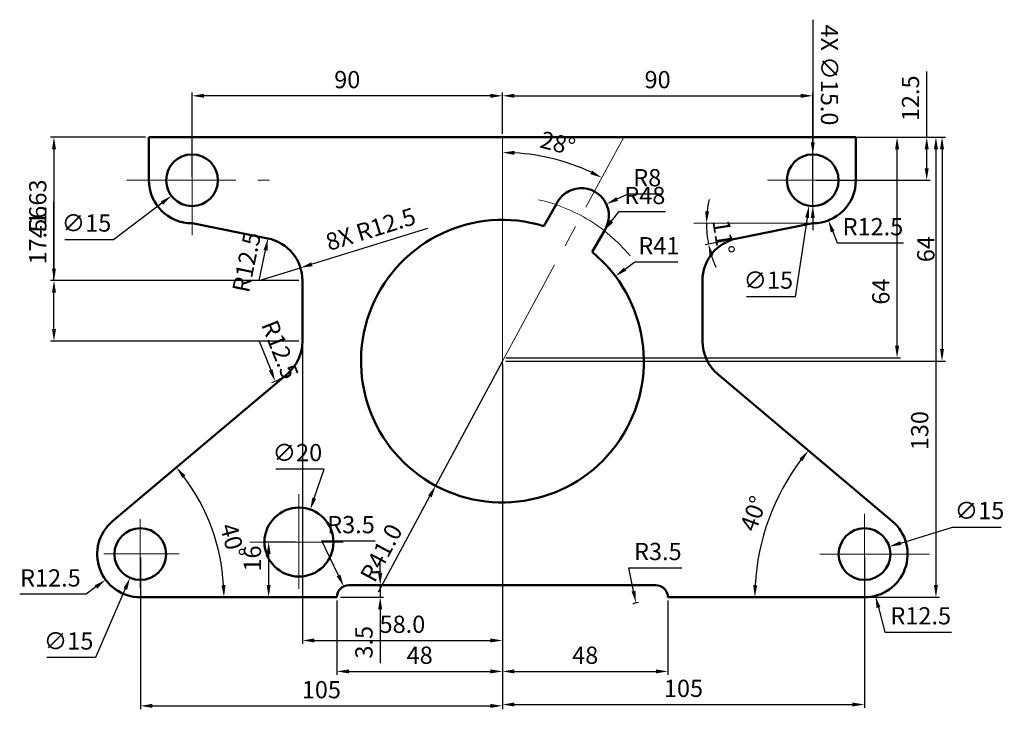
# Model space of a CAD drawing. Units: millimetres. Extents: x 3173 to 3458, y 769 to 969.
import ezdxf

# ---------------------------------------------------------------- set-up
doc = ezdxf.new("R2010")
doc.units = ezdxf.units.MM
doc.linetypes.add('CENTER', pattern=[50.8, 31.75, -6.35, 6.35, -6.35])
for name, color, linetype, lineweight in [('M-CNTR', 7, 'CENTER', 18), ('M-CONS', 8, 'Continuous', 13), ('M-DIMS', 3, 'Continuous', 25), ('M-OUTL', 7, 'Continuous', 50)]:
    doc.layers.add(name, color=color, linetype=linetype, lineweight=lineweight)
doc.styles.get("Standard").update_dxf_attribs({"font": 'arial.ttf'})
doc.dimstyles.new('AM_ISO$0', dxfattribs={"dimtxt": 5, "dimasz": 3.5, "dimexe": 1, "dimexo": 1, "dimgap": 1.5, "dimtad": 1, "dimdsep": 46, "dimtxsty": 'Standard', "dimcen": 0, "dimclrd": 256, "dimclre": 256, "dimclrt": 2, "dimadec": 0, "dimazin": 2, "dimtp": 0.1, "dimtm": 0.1, "dimtfac": 0.71, "dimtmove": 0, "dimatfit": 3, "dimfxl": 1, "dimlwd": -1, "dimlwe": -1, "dimarcsym": 1})
doc.dimstyles.new('AM_ISO$2', dxfattribs={"dimtxt": 5, "dimasz": 3.5, "dimexe": 1, "dimexo": 1, "dimgap": 1.5, "dimtad": 1, "dimdsep": 46, "dimtxsty": 'Standard', "dimcen": 0, "dimclrd": 256, "dimclre": 256, "dimclrt": 2, "dimadec": 0, "dimazin": 2, "dimtp": 0.1, "dimtm": 0.1, "dimtfac": 0.71, "dimtmove": 0, "dimatfit": 3, "dimfxl": 1, "dimlwd": -1, "dimlwe": -1, "dimarcsym": 1})
doc.dimstyles.new('AM_ISO$3', dxfattribs={"dimtxt": 5, "dimasz": 3.5, "dimexe": 1, "dimexo": 1, "dimgap": 1.5, "dimtad": 1, "dimtoh": 1, "dimdsep": 46, "dimtxsty": 'Standard', "dimcen": 0, "dimclrd": 256, "dimclre": 256, "dimclrt": 2, "dimadec": 0, "dimazin": 2, "dimtp": 0.1, "dimtm": 0.1, "dimtfac": 0.71, "dimtofl": 0, "dimtmove": 0, "dimatfit": 0, "dimfxl": 1, "dimlwd": -1, "dimlwe": -1, "dimarcsym": 1})
doc.dimstyles.new('AM_ISO$4', dxfattribs={"dimtxt": 5, "dimasz": 3.5, "dimexe": 1, "dimexo": 1, "dimgap": 1.5, "dimtad": 1, "dimtoh": 1, "dimdsep": 46, "dimtxsty": 'Standard', "dimcen": 0, "dimclrd": 256, "dimclre": 256, "dimclrt": 2, "dimadec": 0, "dimazin": 2, "dimtp": 0.1, "dimtm": 0.1, "dimtfac": 0.71, "dimtofl": 0, "dimtmove": 0, "dimatfit": 0, "dimfxl": 1, "dimlwd": -1, "dimlwe": -1, "dimarcsym": 1})

# ---------------------------------------------------------------- blocks, each defined once
blk = doc.blocks.new('*D3')
at = {"layer": 'Defpoints', "color": 0, "transparency": 16777216}
for p in [(3375.11, 866.04), (3392.94, 831.01), (3425.73, 823.34), (3360.67, 801.29), (3417.67, 801.29)]:
    blk.add_point(p, dxfattribs=at)
at = {"layer": 'M-DIMS', "color": 0, "linetype": 'ByBlock', "transparency": 16777216}
blk.add_arc((3451.87, 801.29), 66, 142.8895, 176.9613, dxfattribs=at)
at = {"layer": 'M-DIMS', "color": 0, "transparency": 16777216}
for points in [[(3398.78, 841.48), (3399.69, 840.75), (3401.42, 843.85)], [(3386.55, 804.77), (3385.38, 804.8), (3385.87, 801.29)]]:
    blk.add_solid(points, dxfattribs=at)
at = {"layer": 'M-DIMS', "color": 0, "transparency": 16777216, "insert": (3386.07, 825.34), "char_height": 5, "attachment_point": 5, "rotation": 69.9254}
blk.add_mtext('40°', dxfattribs=at)
blk = doc.blocks.new('*D4')
at = {"layer": 'Defpoints', "color": 0, "transparency": 16777216}
for p in [(3250.23, 866.04), (3225.65, 827.61), (3199.61, 823.34), (3207.67, 801.29), (3264.67, 801.29)]:
    blk.add_point(p, dxfattribs=at)
at = {"layer": 'M-DIMS', "color": 0, "linetype": 'ByBlock', "transparency": 16777216}
blk.add_arc((3173.46, 801.29), 58.45, 3.4314, 36.7177, dxfattribs=at)
at = {"layer": 'M-DIMS', "color": 0, "transparency": 16777216}
for points in [[(3219.86, 835.87), (3220.77, 836.6), (3218.14, 838.98)], [(3232.39, 804.81), (3231.22, 804.77), (3231.91, 801.29)]]:
    blk.add_solid(points, dxfattribs=at)
at = {"layer": 'M-DIMS', "color": 0, "transparency": 16777216, "insert": (3233.83, 817.5), "char_height": 5, "attachment_point": 5, "rotation": 285.0268}
blk.add_mtext('40°', dxfattribs=at)
blk = doc.blocks.new('*D5')
at = {"layer": 'Defpoints', "color": 0, "transparency": 16777216}
for p in [(3368.19, 909.79), (3402.67, 909.79), (3402.67, 909.79), (3371.9, 907.77), (3380.72, 905.42)]:
    blk.add_point(p, dxfattribs=at)
at = {"layer": 'M-DIMS', "color": 0, "linetype": 'ByBlock', "transparency": 16777216}
blk.add_line((3379.74, 905.22), (3371.44, 903.57), dxfattribs=at)
for start, end in [(166.9868, 173.4934), (180, 191.2657), (197.7723, 204.2789)]:
    blk.add_arc((3402.67, 909.79), 30.84, start, end, dxfattribs=at)
at = {"layer": 'M-DIMS', "color": 0, "transparency": 16777216}
for points in [[(3372.61, 913.25), (3371.45, 913.32), (3371.83, 909.79)], [(3372.74, 900.23), (3373.87, 900.52), (3372.42, 903.77)]]:
    blk.add_solid(points, dxfattribs=at)
at = {"layer": 'M-DIMS', "color": 0, "transparency": 16777216, "insert": (3376.16, 905.64), "char_height": 5, "attachment_point": 5, "rotation": 278.895}
blk.add_mtext('11°', dxfattribs=at)
blk = doc.blocks.new('*D6')
at = {"layer": 'Defpoints', "color": 0, "transparency": 16777216}
for p in [(3244.68, 905.41), (3242.17, 893.16)]:
    blk.add_point(p, dxfattribs=at)
at = {"layer": 'M-DIMS', "color": 0, "linetype": 'ByBlock', "transparency": 16777216}
blk.add_line((3242.17, 893.16), (3243.97, 901.98), dxfattribs=at)
at = {"layer": 'M-DIMS', "color": 0, "transparency": 16777216}
blk.add_solid([(3243.4, 902.09), (3244.55, 901.86), (3244.68, 905.41)], dxfattribs=at)
at = {"layer": 'M-DIMS', "color": 0, "transparency": 16777216, "insert": (3239.1, 898.38), "char_height": 5, "attachment_point": 5, "rotation": 78.4102}
blk.add_mtext('R12.5', dxfattribs=at)
blk = doc.blocks.new('*D7')
at = {"layer": 'Defpoints', "color": 0, "transparency": 16777216}
for p in [(3242.17, 875.6), (3246.75, 863.97)]:
    blk.add_point(p, dxfattribs=at)
at = {"layer": 'M-DIMS', "color": 0, "linetype": 'ByBlock', "transparency": 16777216}
blk.add_line((3242.17, 875.6), (3245.47, 867.23), dxfattribs=at)
blk.add_arc((3242.17, 875.6), 12.5, 286.9476, 305.5655, dxfattribs=at)
at = {"layer": 'M-DIMS', "color": 0, "transparency": 16777216}
blk.add_solid([(3246.01, 867.44), (3244.93, 867.01), (3246.75, 863.97)], dxfattribs=at)
at = {"layer": 'M-DIMS', "color": 0, "transparency": 16777216, "insert": (3247.59, 872.9), "char_height": 5, "attachment_point": 5, "rotation": 291.5312}
blk.add_mtext('R12.5', dxfattribs=at)
blk = doc.blocks.new('*D8')
at = {"layer": 'Defpoints', "color": 0, "transparency": 16777216}
for p in [(3351.39, 799.65), (3352.09, 796.22)]:
    blk.add_point(p, dxfattribs=at)
at = {"layer": 'M-DIMS', "color": 0, "linetype": 'ByBlock', "transparency": 16777216}
for p, q in [((3350.68, 803.07), (3349.28, 809.86)), ((3349.28, 809.86), (3364.7, 809.86))]:
    blk.add_line(p, q, dxfattribs=at)
blk.add_arc((3352.09, 796.22), 3.5, 90, 118.0492, dxfattribs=at)
at = {"layer": 'M-DIMS', "color": 0, "transparency": 16777216}
blk.add_solid([(3351.25, 803.19), (3350.11, 802.96), (3351.39, 799.65)], dxfattribs=at)
at = {"layer": 'M-DIMS', "color": 0, "transparency": 16777216, "insert": (3357.74, 813.91), "char_height": 5, "attachment_point": 5}
blk.add_mtext('R3.5', dxfattribs=at)
blk = doc.blocks.new('*D9')
at = {"layer": 'Defpoints', "color": 0, "transparency": 16777216}
for p in [(3266.65, 804.44), (3268.17, 801.29)]:
    blk.add_point(p, dxfattribs=at)
at = {"layer": 'M-DIMS', "color": 0, "linetype": 'ByBlock', "transparency": 16777216}
for p, q in [((3265.13, 807.6), (3260.3, 817.65)), ((3260.3, 817.65), (3275.73, 817.65))]:
    blk.add_line(p, q, dxfattribs=at)
at = {"layer": 'M-DIMS', "color": 0, "transparency": 16777216}
blk.add_solid([(3265.66, 807.85), (3264.61, 807.35), (3266.65, 804.44)], dxfattribs=at)
at = {"layer": 'M-DIMS', "color": 0, "transparency": 16777216, "insert": (3268.76, 821.7), "char_height": 5, "attachment_point": 5}
blk.add_mtext('R3.5', dxfattribs=at)
blk = doc.blocks.new('*D10')
at = {"layer": 'Defpoints', "color": 0, "transparency": 16777216}
for p in [(3342.79, 915.37), (3335.54, 911.99)]:
    blk.add_point(p, dxfattribs=at)
at = {"layer": 'M-DIMS', "color": 0, "linetype": 'ByBlock', "transparency": 16777216}
for p, q in [((3345.96, 916.85), (3349.14, 918.32)), ((3349.14, 918.32), (3358.71, 918.32))]:
    blk.add_line(p, q, dxfattribs=at)
at = {"layer": 'M-DIMS', "color": 0, "transparency": 16777216}
blk.add_solid([(3345.72, 917.37), (3346.21, 916.32), (3342.79, 915.37)], dxfattribs=at)
at = {"layer": 'M-DIMS', "color": 0, "transparency": 16777216, "insert": (3354.67, 922.38), "char_height": 5, "attachment_point": 5}
blk.add_mtext('R8', dxfattribs=at)
blk = doc.blocks.new('*D11')
at = {"layer": 'Defpoints', "color": 0, "transparency": 16777216}
for p in [(3345.45, 894.41), (3312.67, 869.79)]:
    blk.add_point(p, dxfattribs=at)
at = {"layer": 'M-DIMS', "color": 0, "linetype": 'ByBlock', "transparency": 16777216}
for p, q in [((3348.25, 896.52), (3351.05, 898.62)), ((3351.05, 898.62), (3363.53, 898.62))]:
    blk.add_line(p, q, dxfattribs=at)
at = {"layer": 'M-DIMS', "color": 0, "transparency": 16777216}
blk.add_solid([(3347.9, 896.98), (3348.6, 896.05), (3345.45, 894.41)], dxfattribs=at)
at = {"layer": 'M-DIMS', "color": 0, "transparency": 16777216, "insert": (3358.04, 902.63), "char_height": 5, "attachment_point": 5}
blk.add_mtext('R41', dxfattribs=at)
blk = doc.blocks.new('*D12')
at = {"layer": 'Defpoints', "color": 0, "transparency": 16777216}
for p in [(3342.18, 907.65), (3312.67, 869.79)]:
    blk.add_point(p, dxfattribs=at)
at = {"layer": 'M-DIMS', "color": 0, "linetype": 'ByBlock', "transparency": 16777216}
for p, q in [((3344.33, 910.41), (3346.48, 913.17)), ((3346.48, 913.17), (3359.94, 913.17))]:
    blk.add_line(p, q, dxfattribs=at)
at = {"layer": 'M-DIMS', "color": 0, "transparency": 16777216}
blk.add_solid([(3343.87, 910.77), (3344.79, 910.05), (3342.18, 907.65)], dxfattribs=at)
at = {"layer": 'M-DIMS', "color": 0, "transparency": 16777216, "insert": (3353.96, 917.22), "char_height": 5, "attachment_point": 5}
blk.add_mtext('R48', dxfattribs=at)
blk = doc.blocks.new('*D13')
at = {"layer": 'Defpoints', "color": 0, "transparency": 16777216}
for p in [(3417.67, 813.79), (3420.82, 801.7)]:
    blk.add_point(p, dxfattribs=at)
at = {"layer": 'M-DIMS', "color": 0, "linetype": 'ByBlock', "transparency": 16777216}
for p, q in [((3421.71, 798.31), (3423.57, 791.19)), ((3423.57, 791.19), (3442.88, 791.19))]:
    blk.add_line(p, q, dxfattribs=at)
at = {"layer": 'M-DIMS', "color": 0, "transparency": 16777216}
blk.add_solid([(3422.27, 798.46), (3421.14, 798.16), (3420.82, 801.7)], dxfattribs=at)
at = {"layer": 'M-DIMS', "color": 0, "transparency": 16777216, "insert": (3433.97, 795.25), "char_height": 5, "attachment_point": 5}
blk.add_mtext('R12.5', dxfattribs=at)
blk = doc.blocks.new('*D14')
at = {"layer": 'Defpoints', "color": 0, "transparency": 16777216}
for p in [(3207.67, 813.79), (3197.62, 806.35)]:
    blk.add_point(p, dxfattribs=at)
at = {"layer": 'M-DIMS', "color": 0, "linetype": 'ByBlock', "transparency": 16777216}
for p, q in [((3194.81, 804.27), (3192, 802.19)), ((3192, 802.19), (3172.69, 802.19))]:
    blk.add_line(p, q, dxfattribs=at)
at = {"layer": 'M-DIMS', "color": 0, "transparency": 16777216}
blk.add_solid([(3194.46, 804.74), (3195.16, 803.8), (3197.62, 806.35)], dxfattribs=at)
at = {"layer": 'M-DIMS', "color": 0, "transparency": 16777216, "insert": (3181.59, 806.24), "char_height": 5, "attachment_point": 5}
blk.add_mtext('R12.5', dxfattribs=at)
blk = doc.blocks.new('*D15')
at = {"layer": 'Defpoints', "color": 0, "transparency": 16777216}
for p in [(3402.67, 922.29), (3407.18, 910.63)]:
    blk.add_point(p, dxfattribs=at)
at = {"layer": 'M-DIMS', "color": 0, "linetype": 'ByBlock', "transparency": 16777216}
for p, q in [((3408.44, 907.37), (3409.71, 904.1)), ((3409.71, 904.1), (3429.02, 904.1))]:
    blk.add_line(p, q, dxfattribs=at)
at = {"layer": 'M-DIMS', "color": 0, "transparency": 16777216}
blk.add_solid([(3408.99, 907.58), (3407.9, 907.16), (3407.18, 910.63)], dxfattribs=at)
at = {"layer": 'M-DIMS', "color": 0, "transparency": 16777216, "insert": (3420.11, 908.16), "char_height": 5, "attachment_point": 5}
blk.add_mtext('R12.5', dxfattribs=at)
blk = doc.blocks.new('*D16')
at = {"layer": 'Defpoints', "color": 0, "transparency": 16777216}
for p in [(3402.67, 946.79), (3312.67, 934.79), (3402.67, 922.29)]:
    blk.add_point(p, dxfattribs=at)
at = {"layer": 'M-DIMS', "color": 0, "linetype": 'ByBlock', "transparency": 16777216}
for p, q in [((3312.67, 935.79), (3312.67, 947.79)), ((3316.17, 946.79), (3399.17, 946.79)), ((3402.67, 923.29), (3402.67, 947.79))]:
    blk.add_line(p, q, dxfattribs=at)
at = {"layer": 'M-DIMS', "color": 0, "transparency": 16777216}
for points in [[(3316.17, 947.37), (3316.17, 946.21), (3312.67, 946.79)], [(3399.17, 947.37), (3399.17, 946.21), (3402.67, 946.79)]]:
    blk.add_solid(points, dxfattribs=at)
at = {"layer": 'M-DIMS', "color": 0, "transparency": 16777216, "insert": (3357.67, 950.84), "char_height": 5, "attachment_point": 5}
blk.add_mtext('90', dxfattribs=at)
blk = doc.blocks.new('*D17')
at = {"layer": 'Defpoints', "color": 0, "transparency": 16777216}
for p in [(3222.67, 946.79), (3312.67, 934.79), (3222.67, 922.29)]:
    blk.add_point(p, dxfattribs=at)
at = {"layer": 'M-DIMS', "color": 0, "linetype": 'ByBlock', "transparency": 16777216}
for p, q in [((3222.67, 923.29), (3222.67, 947.79)), ((3309.17, 946.79), (3226.17, 946.79)), ((3312.67, 935.79), (3312.67, 947.79))]:
    blk.add_line(p, q, dxfattribs=at)
at = {"layer": 'M-DIMS', "color": 0, "transparency": 16777216}
for points in [[(3226.17, 947.37), (3226.17, 946.21), (3222.67, 946.79)], [(3309.17, 947.37), (3309.17, 946.21), (3312.67, 946.79)]]:
    blk.add_solid(points, dxfattribs=at)
at = {"layer": 'M-DIMS', "color": 0, "transparency": 16777216, "insert": (3267.67, 950.84), "char_height": 5, "attachment_point": 5}
blk.add_mtext('90', dxfattribs=at)
blk = doc.blocks.new('*D18')
at = {"layer": 'Defpoints', "color": 0, "transparency": 16777216}
for p in [(3256.95, 826.74), (3250.38, 807.84)]:
    blk.add_point(p, dxfattribs=at)
at = {"layer": 'M-DIMS', "color": 0, "linetype": 'ByBlock', "transparency": 16777216}
for p, q in [((3261, 838.41), (3246.92, 838.41)), ((3258.1, 830.04), (3261, 838.41))]:
    blk.add_line(p, q, dxfattribs=at)
at = {"layer": 'M-DIMS', "color": 0, "transparency": 16777216}
blk.add_solid([(3257.55, 830.23), (3258.65, 829.85), (3256.95, 826.74)], dxfattribs=at)
at = {"layer": 'M-DIMS', "color": 0, "transparency": 16777216, "insert": (3253.21, 842.6), "char_height": 5, "attachment_point": 5}
blk.add_mtext('∅20', dxfattribs=at)
blk = doc.blocks.new('*D19')
at = {"layer": 'Defpoints', "color": 0, "transparency": 16777216}
for p in [(3253.67, 817.29), (3244.88, 801.29), (3253.63, 801.29)]:
    blk.add_point(p, dxfattribs=at)
at = {"layer": 'M-DIMS', "color": 0, "linetype": 'ByBlock', "transparency": 16777216}
for p, q in [((3252.67, 817.29), (3243.88, 817.29)), ((3244.88, 813.79), (3244.88, 804.79)), ((3252.63, 801.29), (3243.88, 801.29))]:
    blk.add_line(p, q, dxfattribs=at)
at = {"layer": 'M-DIMS', "color": 0, "transparency": 16777216}
for points in [[(3244.29, 813.79), (3245.46, 813.79), (3244.88, 817.29)], [(3244.29, 804.79), (3245.46, 804.79), (3244.88, 801.29)]]:
    blk.add_solid(points, dxfattribs=at)
at = {"layer": 'M-DIMS', "color": 0, "transparency": 16777216, "insert": (3240.82, 812.52), "char_height": 5, "attachment_point": 5, "rotation": 90}
blk.add_mtext('16', dxfattribs=at)
blk = doc.blocks.new('*D20')
at = {"layer": 'Defpoints', "color": 0, "transparency": 16777216}
for p in [(3271.93, 804.79), (3277.22, 804.79), (3264.67, 801.29)]:
    blk.add_point(p, dxfattribs=at)
at = {"layer": 'M-DIMS', "color": 0, "linetype": 'ByBlock', "transparency": 16777216}
for p, q in [((3277.22, 808.29), (3277.22, 811.79)), ((3272.93, 804.79), (3278.22, 804.79)), ((3277.22, 804.79), (3277.22, 801.29)), ((3265.67, 801.29), (3278.22, 801.29)), ((3277.22, 797.79), (3277.22, 782.15))]:
    blk.add_line(p, q, dxfattribs=at)
at = {"layer": 'M-DIMS', "color": 0, "transparency": 16777216}
for points in [[(3276.63, 808.29), (3277.8, 808.29), (3277.22, 804.79)], [(3276.63, 797.79), (3277.8, 797.79), (3277.22, 801.29)]]:
    blk.add_solid(points, dxfattribs=at)
at = {"layer": 'M-DIMS', "color": 0, "transparency": 16777216, "insert": (3273.16, 788.22), "char_height": 5, "attachment_point": 5, "rotation": 90}
blk.add_mtext('3.5', dxfattribs=at)
blk = doc.blocks.new('*D21')
at = {"layer": 'Defpoints', "color": 0, "transparency": 16777216}
for p in [(3312.67, 804.79), (3360.67, 801.29), (3360.67, 779.76)]:
    blk.add_point(p, dxfattribs=at)
at = {"layer": 'M-DIMS', "color": 0, "linetype": 'ByBlock', "transparency": 16777216}
for p, q in [((3312.67, 803.79), (3312.67, 778.76)), ((3360.67, 800.29), (3360.67, 778.76)), ((3316.17, 779.76), (3357.17, 779.76))]:
    blk.add_line(p, q, dxfattribs=at)
at = {"layer": 'M-DIMS', "color": 0, "transparency": 16777216}
for points in [[(3316.17, 780.34), (3316.17, 779.18), (3312.67, 779.76)], [(3357.17, 780.34), (3357.17, 779.18), (3360.67, 779.76)]]:
    blk.add_solid(points, dxfattribs=at)
at = {"layer": 'M-DIMS', "color": 0, "transparency": 16777216, "insert": (3336.67, 783.81), "char_height": 5, "attachment_point": 5}
blk.add_mtext('48', dxfattribs=at)
blk = doc.blocks.new('*D22')
at = {"layer": 'Defpoints', "color": 0, "transparency": 16777216}
for p in [(3312.67, 804.79), (3264.67, 801.29), (3312.67, 779.76)]:
    blk.add_point(p, dxfattribs=at)
at = {"layer": 'M-DIMS', "color": 0, "linetype": 'ByBlock', "transparency": 16777216}
for p, q in [((3312.67, 803.79), (3312.67, 778.76)), ((3264.67, 800.29), (3264.67, 778.76)), ((3268.17, 779.76), (3309.17, 779.76))]:
    blk.add_line(p, q, dxfattribs=at)
at = {"layer": 'M-DIMS', "color": 0, "transparency": 16777216}
for points in [[(3268.17, 780.34), (3268.17, 779.18), (3264.67, 779.76)], [(3309.17, 780.34), (3309.17, 779.18), (3312.67, 779.76)]]:
    blk.add_solid(points, dxfattribs=at)
at = {"layer": 'M-DIMS', "color": 0, "transparency": 16777216, "insert": (3288.67, 783.81), "char_height": 5, "attachment_point": 5}
blk.add_mtext('48', dxfattribs=at)
blk = doc.blocks.new('*D23')
at = {"layer": 'Defpoints', "color": 0, "transparency": 16777216}
for p in [(3207.67, 813.79), (3312.67, 804.79), (3312.67, 769.76)]:
    blk.add_point(p, dxfattribs=at)
at = {"layer": 'M-DIMS', "color": 0, "linetype": 'ByBlock', "transparency": 16777216}
for p, q in [((3207.67, 812.79), (3207.67, 768.76)), ((3312.67, 803.79), (3312.67, 768.76)), ((3211.17, 769.76), (3309.17, 769.76))]:
    blk.add_line(p, q, dxfattribs=at)
at = {"layer": 'M-DIMS', "color": 0, "transparency": 16777216}
for points in [[(3211.17, 770.34), (3211.17, 769.18), (3207.67, 769.76)], [(3309.17, 770.34), (3309.17, 769.18), (3312.67, 769.76)]]:
    blk.add_solid(points, dxfattribs=at)
at = {"layer": 'M-DIMS', "color": 0, "transparency": 16777216, "insert": (3260.17, 773.81), "char_height": 5, "attachment_point": 5}
blk.add_mtext('105', dxfattribs=at)
blk = doc.blocks.new('*D24')
at = {"layer": 'Defpoints', "color": 0, "transparency": 16777216}
for p in [(3417.67, 813.79), (3312.67, 804.79), (3417.67, 770.15)]:
    blk.add_point(p, dxfattribs=at)
at = {"layer": 'M-DIMS', "color": 0, "linetype": 'ByBlock', "transparency": 16777216}
for p, q in [((3417.67, 812.79), (3417.67, 769.15)), ((3312.67, 803.79), (3312.67, 769.15)), ((3316.17, 770.15), (3414.17, 770.15))]:
    blk.add_line(p, q, dxfattribs=at)
at = {"layer": 'M-DIMS', "color": 0, "transparency": 16777216}
for points in [[(3316.17, 770.73), (3316.17, 769.57), (3312.67, 770.15)], [(3414.17, 770.73), (3414.17, 769.57), (3417.67, 770.15)]]:
    blk.add_solid(points, dxfattribs=at)
at = {"layer": 'M-DIMS', "color": 0, "transparency": 16777216, "insert": (3365.17, 774.2), "char_height": 5, "attachment_point": 5}
blk.add_mtext('105', dxfattribs=at)
blk = doc.blocks.new('*D25')
at = {"layer": 'Defpoints', "color": 0, "transparency": 16777216}
for p in [(3415.17, 934.79), (3312.67, 869.79), (3440.14, 869.79)]:
    blk.add_point(p, dxfattribs=at)
at = {"layer": 'M-DIMS', "color": 0, "linetype": 'ByBlock', "transparency": 16777216}
for p, q in [((3416.17, 934.79), (3441.14, 934.79)), ((3440.14, 931.29), (3440.14, 873.29)), ((3313.67, 869.79), (3441.14, 869.79))]:
    blk.add_line(p, q, dxfattribs=at)
at = {"layer": 'M-DIMS', "color": 0, "transparency": 16777216}
for points in [[(3439.56, 931.29), (3440.72, 931.29), (3440.14, 934.79)], [(3439.56, 873.29), (3440.72, 873.29), (3440.14, 869.79)]]:
    blk.add_solid(points, dxfattribs=at)
at = {"layer": 'M-DIMS', "color": 0, "transparency": 16777216, "insert": (3436.09, 902.29), "char_height": 5, "attachment_point": 5, "rotation": 90}
blk.add_mtext('64', dxfattribs=at)
blk = doc.blocks.new('*D26')
at = {"layer": 'Defpoints', "color": 0, "transparency": 16777216}
for p in [(3415.17, 934.79), (3427.11, 934.79), (3312.67, 870.79)]:
    blk.add_point(p, dxfattribs=at)
at = {"layer": 'M-DIMS', "color": 0, "linetype": 'ByBlock', "transparency": 16777216}
for p, q in [((3416.17, 934.79), (3428.11, 934.79)), ((3427.11, 874.29), (3427.11, 931.29)), ((3313.67, 870.79), (3428.11, 870.79))]:
    blk.add_line(p, q, dxfattribs=at)
at = {"layer": 'M-DIMS', "color": 0, "transparency": 16777216}
for points in [[(3426.53, 931.29), (3427.7, 931.29), (3427.11, 934.79)], [(3426.53, 874.29), (3427.7, 874.29), (3427.11, 870.79)]]:
    blk.add_solid(points, dxfattribs=at)
at = {"layer": 'M-DIMS', "color": 0, "transparency": 16777216, "insert": (3423.06, 889.97), "char_height": 5, "attachment_point": 5, "rotation": 90}
blk.add_mtext('64', dxfattribs=at)
blk = doc.blocks.new('*D27')
at = {"layer": 'Defpoints', "color": 0, "transparency": 16777216}
for p in [(3415.17, 934.79), (3407.81, 801.29), (3438.38, 801.29)]:
    blk.add_point(p, dxfattribs=at)
at = {"layer": 'M-DIMS', "color": 0, "linetype": 'ByBlock', "transparency": 16777216}
for p, q in [((3416.17, 934.79), (3439.38, 934.79)), ((3438.38, 931.29), (3438.38, 804.79)), ((3408.81, 801.29), (3439.38, 801.29))]:
    blk.add_line(p, q, dxfattribs=at)
at = {"layer": 'M-DIMS', "color": 0, "transparency": 16777216}
for points in [[(3437.79, 931.29), (3438.96, 931.29), (3438.38, 934.79)], [(3437.79, 804.79), (3438.96, 804.79), (3438.38, 801.29)]]:
    blk.add_solid(points, dxfattribs=at)
at = {"layer": 'M-DIMS', "color": 0, "transparency": 16777216, "insert": (3434.32, 849.62), "char_height": 5, "attachment_point": 5, "rotation": 90}
blk.add_mtext('130', dxfattribs=at)
blk = doc.blocks.new('*D28')
at = {"layer": 'Defpoints', "color": 0, "transparency": 16777216}
for p in [(3402.67, 934.79), (3435.7, 934.79), (3402.67, 922.29)]:
    blk.add_point(p, dxfattribs=at)
at = {"layer": 'M-DIMS', "color": 0, "linetype": 'ByBlock', "transparency": 16777216}
for p, q in [((3435.7, 934.79), (3435.7, 953.84)), ((3403.67, 934.79), (3436.7, 934.79)), ((3435.7, 925.79), (3435.7, 931.29)), ((3403.67, 922.29), (3436.7, 922.29))]:
    blk.add_line(p, q, dxfattribs=at)
at = {"layer": 'M-DIMS', "color": 0, "transparency": 16777216}
for points in [[(3435.12, 931.29), (3436.29, 931.29), (3435.7, 934.79)], [(3435.12, 925.79), (3436.29, 925.79), (3435.7, 922.29)]]:
    blk.add_solid(points, dxfattribs=at)
at = {"layer": 'M-DIMS', "color": 0, "transparency": 16777216, "insert": (3431.65, 946.07), "char_height": 5, "attachment_point": 5, "rotation": 90}
blk.add_mtext('12.5', dxfattribs=at)
blk = doc.blocks.new('*D29')
at = {"layer": 'Defpoints', "color": 0, "transparency": 16777216}
for p in [(3312.67, 934.79), (3347.9, 934.79), (3322.64, 929.5), (3312.67, 870.79), (3312.67, 869.79)]:
    blk.add_point(p, dxfattribs=at)
at = {"layer": 'M-DIMS', "color": 0, "linetype": 'ByBlock', "transparency": 16777216}
blk.add_arc((3312.67, 869.79), 60.54, 64.8556, 86.6871, dxfattribs=at)
at = {"layer": 'M-DIMS', "color": 0, "transparency": 16777216}
for points in [[(3316.15, 929.65), (3316.18, 930.81), (3312.67, 930.33)], [(3338.65, 925.11), (3338.13, 924.07), (3341.51, 923.02)]]:
    blk.add_solid(points, dxfattribs=at)
at = {"layer": 'M-DIMS', "color": 0, "transparency": 16777216, "insert": (3328.57, 932.4), "char_height": 5, "attachment_point": 5, "rotation": 345.7448}
blk.add_mtext('28°', dxfattribs=at)
blk = doc.blocks.new('*D30')
at = {"layer": 'Defpoints', "color": 0, "transparency": 16777216}
for p in [(3210.64, 820.67), (3204.69, 806.91)]:
    blk.add_point(p, dxfattribs=at)
at = {"layer": 'M-DIMS', "color": 0, "linetype": 'ByBlock', "transparency": 16777216}
for p, q in [((3203.3, 803.69), (3194.68, 783.76)), ((3194.68, 783.76), (3180.54, 783.76))]:
    blk.add_line(p, q, dxfattribs=at)
at = {"layer": 'M-DIMS', "color": 0, "transparency": 16777216}
blk.add_solid([(3202.77, 803.93), (3203.84, 803.46), (3204.69, 806.91)], dxfattribs=at)
at = {"layer": 'M-DIMS', "color": 0, "transparency": 16777216, "insert": (3186.86, 787.95), "char_height": 5, "attachment_point": 5}
blk.add_mtext('∅15', dxfattribs=at)
blk = doc.blocks.new('*D31')
at = {"layer": 'Defpoints', "color": 0, "transparency": 16777216}
for p in [(3228.65, 926.82), (3216.69, 917.76)]:
    blk.add_point(p, dxfattribs=at)
at = {"layer": 'M-DIMS', "color": 0, "linetype": 'ByBlock', "transparency": 16777216}
for p, q in [((3213.89, 915.65), (3199.87, 905.04)), ((3199.87, 905.04), (3185.73, 905.04))]:
    blk.add_line(p, q, dxfattribs=at)
at = {"layer": 'M-DIMS', "color": 0, "transparency": 16777216}
blk.add_solid([(3213.54, 916.12), (3214.25, 915.19), (3216.69, 917.76)], dxfattribs=at)
at = {"layer": 'M-DIMS', "color": 0, "transparency": 16777216, "insert": (3192.05, 909.23), "char_height": 5, "attachment_point": 5}
blk.add_mtext('∅15', dxfattribs=at)
blk = doc.blocks.new('*D32')
at = {"layer": 'Defpoints', "color": 0, "transparency": 16777216}
for p in [(3403.78, 929.71), (3401.55, 914.87)]:
    blk.add_point(p, dxfattribs=at)
at = {"layer": 'M-DIMS', "color": 0, "linetype": 'ByBlock', "transparency": 16777216}
for p, q in [((3401.04, 911.41), (3397.59, 888.45)), ((3397.59, 888.45), (3383.45, 888.45))]:
    blk.add_line(p, q, dxfattribs=at)
at = {"layer": 'M-DIMS', "color": 0, "transparency": 16777216}
blk.add_solid([(3400.46, 911.5), (3401.61, 911.33), (3401.55, 914.87)], dxfattribs=at)
at = {"layer": 'M-DIMS', "color": 0, "transparency": 16777216, "insert": (3389.77, 892.65), "char_height": 5, "attachment_point": 5}
blk.add_mtext('∅15', dxfattribs=at)
blk = doc.blocks.new('*D33')
at = {"layer": 'Defpoints', "color": 0, "transparency": 16777216}
for p in [(3424.84, 815.98), (3410.49, 811.6)]:
    blk.add_point(p, dxfattribs=at)
at = {"layer": 'M-DIMS', "color": 0, "linetype": 'ByBlock', "transparency": 16777216}
for p, q in [((3428.19, 817.01), (3443.19, 821.59)), ((3443.19, 821.59), (3457.33, 821.59))]:
    blk.add_line(p, q, dxfattribs=at)
at = {"layer": 'M-DIMS', "color": 0, "transparency": 16777216}
blk.add_solid([(3428.02, 817.56), (3428.36, 816.45), (3424.84, 815.98)], dxfattribs=at)
at = {"layer": 'M-DIMS', "color": 0, "transparency": 16777216, "insert": (3451.01, 825.79), "char_height": 5, "attachment_point": 5}
blk.add_mtext('∅15', dxfattribs=at)
blk = doc.blocks.new('MOUNT-HOLE-D15')
blk.add_circle((0, 0), 7.5)
blk = doc.blocks.new('*D35')
at = {"layer": 'Defpoints', "color": 0, "transparency": 16777216}
for p in [(3254.67, 875.6), (3312.67, 869.79), (3312.67, 788.74)]:
    blk.add_point(p, dxfattribs=at)
at = {"layer": 'M-DIMS', "linetype": 'ByBlock', "transparency": 16777216}
for p, q in [((3254.67, 874.6), (3254.67, 787.74)), ((3312.67, 868.79), (3312.67, 787.74)), ((3258.17, 788.74), (3309.17, 788.74))]:
    blk.add_line(p, q, dxfattribs=at)
at = {"layer": 'M-DIMS', "transparency": 16777216}
for points in [[(3258.17, 789.32), (3258.17, 788.16), (3254.67, 788.74)], [(3309.17, 789.32), (3309.17, 788.16), (3312.67, 788.74)]]:
    blk.add_solid(points, dxfattribs=at)
at = {"layer": 'M-DIMS', "color": 2, "transparency": 16777216, "insert": (3283.67, 792.79), "char_height": 5, "attachment_point": 5}
blk.add_mtext('58.0', dxfattribs=at)
blk = doc.blocks.new('*D36')
at = {"layer": 'Defpoints', "color": 0, "transparency": 16777216}
for p in [(3182.63, 893.16), (3254.67, 893.16), (3254.67, 875.6)]:
    blk.add_point(p, dxfattribs=at)
at = {"layer": 'M-DIMS', "linetype": 'ByBlock', "transparency": 16777216}
for p, q in [((3182.63, 893.16), (3182.63, 916.06)), ((3253.67, 893.16), (3181.63, 893.16)), ((3182.63, 879.1), (3182.63, 889.66)), ((3253.67, 875.6), (3181.63, 875.6))]:
    blk.add_line(p, q, dxfattribs=at)
at = {"layer": 'M-DIMS', "transparency": 16777216}
for points in [[(3182.04, 889.66), (3183.21, 889.66), (3182.63, 893.16)], [(3182.04, 879.1), (3183.21, 879.1), (3182.63, 875.6)]]:
    blk.add_solid(points, dxfattribs=at)
at = {"layer": 'M-DIMS', "color": 2, "transparency": 16777216, "insert": (3178.57, 906.36), "char_height": 5, "attachment_point": 5, "rotation": 90}
blk.add_mtext('17.56', dxfattribs=at)
blk = doc.blocks.new('*D37')
at = {"layer": 'Defpoints', "color": 0, "transparency": 16777216}
for p in [(3210.17, 934.79), (3182.63, 893.16), (3254.67, 893.16)]:
    blk.add_point(p, dxfattribs=at)
at = {"layer": 'M-DIMS', "linetype": 'ByBlock', "transparency": 16777216}
for p, q in [((3209.17, 934.79), (3181.63, 934.79)), ((3182.63, 931.29), (3182.63, 896.66)), ((3253.67, 893.16), (3181.63, 893.16))]:
    blk.add_line(p, q, dxfattribs=at)
at = {"layer": 'M-DIMS', "transparency": 16777216}
for points in [[(3182.04, 931.29), (3183.21, 931.29), (3182.63, 934.79)], [(3182.04, 896.66), (3183.21, 896.66), (3182.63, 893.16)]]:
    blk.add_solid(points, dxfattribs=at)
at = {"layer": 'M-DIMS', "color": 2, "transparency": 16777216, "insert": (3178.57, 913.98), "char_height": 5, "attachment_point": 5, "rotation": 90}
blk.add_mtext('41.63', dxfattribs=at)
blk = doc.blocks.new('*D38')
at = {"layer": 'Defpoints', "color": 0, "transparency": 16777216}
for p in [(3312.67, 869.79), (3293.3, 833.65)]:
    blk.add_point(p, dxfattribs=at)
at = {"layer": 'M-DIMS', "linetype": 'ByBlock', "transparency": 16777216}
for p, q in [((3312.67, 869.79), (3293.3, 833.65)), ((3276.78, 802.82), (3291.65, 830.57))]:
    blk.add_line(p, q, dxfattribs=at)
at = {"layer": 'M-DIMS', "transparency": 16777216}
blk.add_solid([(3291.13, 830.84), (3292.16, 830.29), (3293.3, 833.65)], dxfattribs=at)
at = {"layer": 'M-DIMS', "color": 2, "transparency": 16777216, "insert": (3278.11, 813.88), "char_height": 5, "attachment_point": 5, "rotation": 61.8163}
blk.add_mtext('R41.0', dxfattribs=at)
blk = doc.blocks.new('*D39')
at = {"layer": 'Defpoints', "color": 0, "transparency": 16777216}
for p in [(3254.1, 896.87), (3242.17, 893.16)]:
    blk.add_point(p, dxfattribs=at)
at = {"layer": 'M-DIMS', "linetype": 'ByBlock', "transparency": 16777216}
for p, q in [((3290.93, 908.3), (3257.45, 897.91)), ((3242.17, 893.16), (3254.1, 896.87))]:
    blk.add_line(p, q, dxfattribs=at)
at = {"layer": 'M-DIMS', "transparency": 16777216}
blk.add_solid([(3257.27, 898.46), (3257.62, 897.35), (3254.1, 896.87)], dxfattribs=at)
at = {"layer": 'M-DIMS', "color": 2, "transparency": 16777216, "insert": (3274.66, 907.49), "char_height": 5, "attachment_point": 5, "rotation": 17.2503}
blk.add_mtext('8X R12.5', dxfattribs=at)
blk = doc.blocks.new('*D40')
at = {"layer": 'Defpoints', "color": 0, "transparency": 16777216}
for p in [(3402.67, 929.79), (3402.67, 914.79)]:
    blk.add_point(p, dxfattribs=at)
at = {"layer": 'M-DIMS', "linetype": 'ByBlock', "transparency": 16777216}
for p, q in [((3402.66, 968.88), (3402.67, 933.29)), ((3402.67, 914.79), (3402.67, 929.79)), ((3402.67, 911.29), (3402.67, 907.79))]:
    blk.add_line(p, q, dxfattribs=at)
at = {"layer": 'M-DIMS', "transparency": 16777216}
for points in [[(3403.25, 933.29), (3402.08, 933.29), (3402.67, 929.79)], [(3403.25, 911.29), (3402.08, 911.29), (3402.67, 914.79)]]:
    blk.add_solid(points, dxfattribs=at)
at = {"layer": 'M-DIMS', "color": 2, "transparency": 16777216, "insert": (3406.86, 952.84), "char_height": 5, "attachment_point": 5, "rotation": 270.0037}
blk.add_mtext('4X ∅15.0', dxfattribs=at)

msp = doc.modelspace()

# ---------------------------------------------------------------- linework, layer by layer
at = {"layer": 'M-CNTR'}
for p, q in [((3222.666, 938.113), (3222.666, 904.742)), ((3312.666, 804.79), (3312.666, 934.79)), ((3312.666, 869.79), (3347.896, 934.79)), ((3402.666, 934.79), (3402.666, 912.21)), ((3203.62, 922.29), (3245.152, 922.29)), ((3389.51, 922.29), (3413.852, 922.29)), ((3253.666, 831.154), (3253.666, 803.767)), ((3417.666, 825.445), (3417.666, 801.29)), ((3207.666, 823.95), (3207.666, 803.882)), ((3266.485, 817.29), (3239.417, 817.29)), ((3218.946, 813.916), (3197.079, 813.916)), ((3436.488, 813.79), (3403.376, 813.79))]:
    msp.add_line(p, q, dxfattribs=at)
msp.add_arc((3312.666, 869.79), 48, 39.50874, 79.33791, dxfattribs=at)
msp.add_arc((3312.666, 869.79), 48, 39.50874, 79.33791, dxfattribs=at)
at = {"layer": 'M-CONS'}
for p, q in [((3312.666, 934.79), (3312.666, 870.79)), ((3321.547, 916.962), (3321.547, 916.962)), ((3402.666, 909.79), (3368.187, 909.79)), ((3264.666, 801.29), (3264.666, 801.29)), ((3360.666, 801.29), (3360.666, 801.29))]:
    msp.add_line(p, q, dxfattribs=at)
at = {"layer": 'M-OUTL'}
for p, q in [((3222.666, 934.79), (3210.166, 934.79)), ((3210.166, 922.29), (3210.166, 934.79)), ((3312.666, 934.79), (3222.666, 934.79)), ((3312.666, 934.79), (3402.666, 934.79)), ((3402.666, 934.79), (3415.166, 934.79)), ((3415.166, 922.29), (3415.166, 934.79)), ((3328.212, 915.203), (3324.633, 909.005)), ((3222.666, 909.79), (3244.608, 905.419)), ((3402.666, 909.79), (3380.725, 905.419)), ((3342.23, 907.606), (3338.689, 901.473)), ((3254.666, 875.599), (3254.666, 893.16)), ((3370.666, 875.599), (3370.666, 893.16)), ((3250.226, 866.045), (3199.607, 823.345)), ((3375.107, 866.045), (3425.726, 823.345)), ((3268.166, 804.79), (3312.666, 804.79)), ((3312.666, 804.79), (3357.166, 804.79)), ((3264.666, 801.29), (3207.666, 801.29)), ((3360.666, 801.29), (3417.666, 801.29))]:
    msp.add_line(p, q, dxfattribs=at)
for centre, radius in [((3222.666, 922.29), 7.5), ((3253.666, 817.29), 10), ((3207.666, 813.79), 7.5)]:
    msp.add_circle(centre, radius, dxfattribs=at)
for centre, radius, start, end in [((3222.666, 922.29), 12.5, 180, 270), ((3402.666, 922.29), 12.5, 270, 0), ((3335.539, 911.991), 8, 326.76257, 156.32295), ((3312.666, 869.79), 41, 73.02961, 50.60204), ((3242.166, 893.16), 12.5, 0, 78.73432), ((3383.166, 893.16), 12.5, 101.26568, 180), ((3242.166, 875.599), 12.5, 310.14915, 0), ((3383.166, 875.599), 12.5, 180, 229.85085), ((3207.666, 813.79), 12.5, 130.14915, 270), ((3207.666, 813.79), 12.5, 130.14915, 270), ((3417.666, 813.79), 12.5, 270, 49.85085), ((3268.166, 801.29), 3.5, 90, 180), ((3357.166, 801.29), 3.5, 0, 90)]:
    msp.add_arc(centre, radius, start, end, dxfattribs=at)

# ---------------------------------------------------------------- block references
for p in [(3222.666, 922.29), (3402.666, 922.29), (3207.666, 813.79), (3417.666, 813.79)]:
    msp.add_blockref('MOUNT-HOLE-D15', p, dxfattribs=at)

# ---------------------------------------------------------------- dimensions: what is measured, and where the dimension line sits
at = {"layer": 'M-DIMS'}
dim = msp.add_diameter_dim_2p(p1=(3402.667, 914.79), p2=(3402.666, 929.79), text='4X <>', dimstyle='AM_ISO$0', override={"dimdec": 1, "dimlfac": 1, "dimrnd": 0, "dimzin": 0, "dimdsep": 46, "dimlunit": 2}, dxfattribs=at)
dim.commit()
dim.dimension.update_dxf_attribs({"geometry": '*D40', "text_midpoint": (3402.664, 952.835)})
for base, p1, p2, override, picture, middle in [((3222.666, 946.79), (3312.666, 934.79), (3222.666, 922.29), {"dimclrd": 0, "dimclre": 0, "dimclrt": 0}, '*D17', (3267.666, 950.843)), ((3402.666, 946.79), (3312.666, 934.79), (3402.666, 922.29), {"dimpost": '', "dimclrd": 0, "dimclre": 0, "dimclrt": 0}, '*D16', (3357.666, 950.843)), ((3312.666, 788.74), (3254.666, 875.599), (3312.666, 869.79), {"dimdec": 1, "dimlfac": 1, "dimrnd": 0, "dimzin": 0, "dimdsep": 46, "dimlunit": 2}, '*D35', (3283.666, 792.793))]:
    dim = msp.add_linear_dim(base=base, p1=p1, p2=p2, dimstyle='AM_ISO$0', override=override, dxfattribs=at)
    dim.commit()
    dim.dimension.update_dxf_attribs({"geometry": picture, "text_midpoint": middle})
for base, p1, p2, angle, override, picture, middle in [((3435.703, 934.79), (3402.666, 922.29), (3402.666, 934.79), 90, {"dimpost": '', "dimclrd": 0, "dimclre": 0, "dimclrt": 0}, '*D28', (3431.65, 946.068)), ((3182.627, 893.16), (3210.166, 934.79), (3254.666, 893.16), 90, {"dimdec": 2, "dimlfac": 1, "dimrnd": 0, "dimzin": 0, "dimdsep": 46, "dimlunit": 2}, '*D37', (3178.572, 913.975)), ((3182.627, 893.16), (3254.666, 875.599), (3254.666, 893.16), 90, {"dimdec": 2, "dimlfac": 1, "dimrnd": 0, "dimzin": 0, "dimdsep": 46, "dimlunit": 2}, '*D36', (3178.574, 906.36)), ((3312.666, 769.759), (3207.666, 813.79), (3312.666, 804.79), 0, {"dimclrd": 0, "dimclre": 0, "dimclrt": 0}, '*D23', (3260.166, 773.812)), ((3417.666, 770.15), (3312.666, 804.79), (3417.666, 813.79), 0, {"dimclrd": 0, "dimclre": 0, "dimclrt": 0}, '*D24', (3365.166, 774.203)), ((3312.666, 779.759), (3264.666, 801.29), (3312.666, 804.79), 0, {"dimclrd": 0, "dimclre": 0, "dimclrt": 0}, '*D22', (3288.666, 783.812)), ((3360.666, 779.759), (3312.666, 804.79), (3360.666, 801.29), 0, {"dimpost": '', "dimclrd": 0, "dimclre": 0, "dimclrt": 0}, '*D21', (3336.666, 783.812))]:
    dim = msp.add_linear_dim(base=base, p1=p1, p2=p2, angle=angle, dimstyle='AM_ISO$0', override=override, dxfattribs=at)
    dim.commit()
    dim.dimension.update_dxf_attribs({"geometry": picture, "text_midpoint": middle})
for base, line1, line2, picture, middle in [((3322.644, 929.503), ((3312.666, 934.79), (3312.666, 870.79)), ((3312.666, 869.79), (3347.896, 934.79)), '*D29', (3327.574, 928.467)), ((3371.896, 907.771), ((3402.666, 909.79), (3368.187, 909.79)), ((3402.666, 909.79), (3380.725, 905.419)), '*D5', (3372.2, 905.022)), ((3225.648, 827.613), ((3250.226, 866.045), (3199.607, 823.345)), ((3264.666, 801.29), (3207.666, 801.29)), '*D4', (3229.912, 816.445))]:
    dim = msp.add_angular_dim_2l(base=base, line1=line1, line2=line2, dimstyle='AM_ISO$2', override={"dimclrd": 0, "dimclre": 0, "dimclrt": 0}, dxfattribs=at)
    dim.commit()
    dim.dimension.update_dxf_attribs({"geometry": picture, "text_midpoint": middle, "dimtype": 162})
dim = msp.add_linear_dim(base=(3440.139, 869.79), p1=(3415.166, 934.79), p2=(3312.666, 869.79), angle=90, text='64', dimstyle='AM_ISO$0', override={"dimpost": '', "dimclrd": 0, "dimclre": 0, "dimclrt": 0}, dxfattribs=at)
dim.commit()
dim.dimension.update_dxf_attribs({"geometry": '*D25', "text_midpoint": (3436.086, 902.29)})
for base, p1, p2, picture, middle in [((3427.113, 934.79), (3312.666, 870.79), (3415.166, 934.79), '*D26', (3427.113, 889.974)), ((3244.876, 801.29), (3253.666, 817.29), (3253.627, 801.29), '*D19', (3244.876, 812.523)), ((3277.217, 804.79), (3264.666, 801.29), (3271.935, 804.79), '*D20', (3277.217, 788.222))]:
    dim = msp.add_linear_dim(base=base, p1=p1, p2=p2, angle=90, dimstyle='AM_ISO$0', override={"dimclrd": 0, "dimclre": 0, "dimclrt": 0}, dxfattribs=at)
    dim.commit()
    dim.dimension.update_dxf_attribs({"geometry": picture, "text_midpoint": middle, "dimtype": 160})
dim = msp.add_linear_dim(base=(3438.377, 801.29), p1=(3415.166, 934.79), p2=(3407.813, 801.29), angle=90, text='130', dimstyle='AM_ISO$0', override={"dimclrd": 0, "dimclre": 0, "dimclrt": 0}, dxfattribs=at)
dim.commit()
dim.dimension.update_dxf_attribs({"geometry": '*D27', "text_midpoint": (3438.377, 849.618), "dimtype": 160})
for p1, p2, override, picture, middle in [((3403.779, 929.707), (3401.554, 914.873), {"dimclrd": 0, "dimclre": 0, "dimclrt": 0}, '*D32', (3389.772, 888.454)), ((3228.647, 926.816), (3216.686, 917.765), {"dimclrd": 0, "dimclre": 0, "dimclrt": 0}, '*D31', (3192.05, 905.039)), ((3250.384, 807.844), (3256.949, 826.736), {"dimpost": '', "dimclrd": 0, "dimclre": 0, "dimclrt": 0}, '*D18', (3253.212, 838.407)), ((3410.494, 811.597), (3424.839, 815.983), {"dimclrd": 0, "dimclre": 0, "dimclrt": 0}, '*D33', (3451.009, 821.594)), ((3210.643, 820.674), (3204.69, 806.906), {"dimpost": '', "dimclrd": 0, "dimclre": 0, "dimclrt": 0}, '*D30', (3186.861, 783.758))]:
    dim = msp.add_diameter_dim_2p(p1=p1, p2=p2, dimstyle='AM_ISO$3', override=override, dxfattribs=at)
    dim.commit()
    dim.dimension.update_dxf_attribs({"geometry": picture, "text_midpoint": middle, "dimtype": 163})
for center, mpoint, dimstyle, override, picture, middle in [((3335.539, 911.991), (3342.791, 915.368), 'AM_ISO$4', {"dimclrd": 0, "dimclre": 0, "dimclrt": 0}, '*D10', (3354.673, 918.323)), ((3402.666, 922.29), (3407.178, 910.633), 'AM_ISO$4', {"dimclrd": 0, "dimclre": 0, "dimclrt": 0}, '*D15', (3420.11, 904.105)), ((3312.666, 869.79), (3342.177, 907.647), 'AM_ISO$4', {"dimclrd": 0, "dimclre": 0, "dimclrt": 0}, '*D12', (3353.96, 913.167)), ((3242.166, 893.16), (3244.678, 905.405), 'AM_ISO$4', {"dimpost": '', "dimclrd": 0, "dimclre": 0, "dimclrt": 0}, '*D6', (3243.071, 897.569)), ((3312.666, 869.79), (3345.448, 894.414), 'AM_ISO$4', {"dimclrd": 0, "dimclre": 0, "dimclrt": 0}, '*D11', (3358.036, 898.618)), ((3242.166, 875.599), (3246.754, 863.972), 'AM_ISO$4', {"dimclrd": 0, "dimclre": 0, "dimclrt": 0}, '*D7', (3243.818, 871.413)), ((3312.666, 869.79), (3293.302, 833.651), 'AM_ISO$0', {"dimdec": 1, "dimlfac": 1, "dimrnd": 0, "dimzin": 0, "dimdsep": 46, "dimlunit": 2}, '*D38', (3281.684, 811.968)), ((3268.166, 801.29), (3266.65, 804.445), 'AM_ISO$4', {"dimclrd": 0, "dimclre": 0, "dimclrt": 0}, '*D9', (3268.763, 817.649)), ((3352.094, 796.218), (3351.386, 799.646), 'AM_ISO$4', {"dimclrd": 0, "dimclre": 0, "dimclrt": 0}, '*D8', (3357.738, 809.856)), ((3207.666, 813.79), (3197.621, 806.351), 'AM_ISO$4', {"dimclrd": 0, "dimclre": 0, "dimclrt": 0}, '*D14', (3181.59, 802.186)), ((3417.666, 813.79), (3420.824, 801.696), 'AM_ISO$4', {"dimclrd": 0, "dimclre": 0, "dimclrt": 0}, '*D13', (3433.97, 791.195))]:
    dim = msp.add_radius_dim(center=center, mpoint=mpoint, dimstyle=dimstyle, override=override, dxfattribs=at)
    dim.commit()
    dim.dimension.update_dxf_attribs({"geometry": picture, "text_midpoint": middle, "dimtype": 164})
dim = msp.add_radius_dim(center=(3242.166, 893.16), mpoint=(3254.104, 896.867), text='8X <>', dimstyle='AM_ISO$0', override={"dimdec": 1, "dimlfac": 1, "dimrnd": 0, "dimzin": 0, "dimdsep": 46, "dimlunit": 2}, dxfattribs=at)
dim.commit()
dim.dimension.update_dxf_attribs({"geometry": '*D39', "text_midpoint": (3274.658, 907.493)})
dim = msp.add_angular_dim_2l(base=(3392.941, 831.014), line1=((3375.107, 866.045), (3425.726, 823.345)), line2=((3360.666, 801.29), (3417.666, 801.29)), dimstyle='AM_ISO$2', override={"dimpost": '', "dimclrd": 0, "dimclre": 0, "dimclrt": 0}, dxfattribs=at)
dim.commit()
dim.dimension.update_dxf_attribs({"geometry": '*D3', "text_midpoint": (3386.073, 825.336)})

doc.saveas('drawing.dxf')
